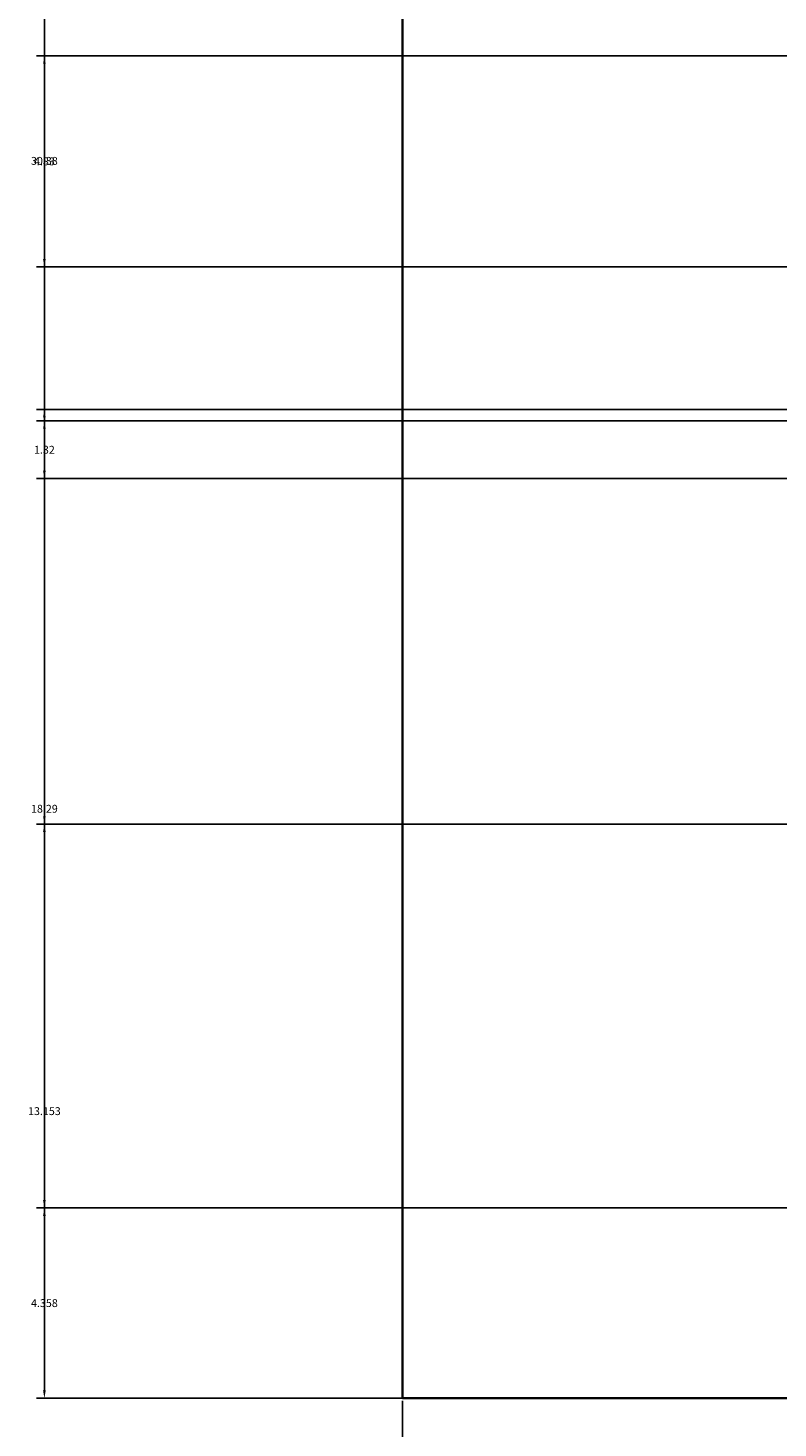
# Model space of a CAD drawing. Units: inches. Extents: x 27 to 200, y -50 to 102.
# Tile 2 of 26: x 27 to 44, y -17 to 15. Entities that reach past the tile are written whole.
import ezdxf

# ---------------------------------------------------------------- set-up
doc = ezdxf.new("R2010")
doc.units = ezdxf.units.IN
doc.header["$MEASUREMENT"] = 0
doc.layers.add('A-ANNO-DIMS', color=2, linetype='Continuous', lineweight=18)
doc.layers.add('A-ELEV', color=7, linetype='Continuous', lineweight=35)
doc.styles.get("Standard").update_dxf_attribs({"font": 'arial.ttf'})
doc.dimstyles.get("Standard").update_dxf_attribs({"dimtxt": 0.18, "dimasz": 0.18, "dimexe": 0.18, "dimexo": 0.0625, "dimgap": 0.09, "dimtad": 0, "dimtih": 1, "dimtoh": 1, "dimdec": 4, "dimzin": 0, "dimdsep": 46, "dimtxsty": 'Standard', "dimcen": 0.09, "dimadec": 0, "dimazin": 0, "dimtfac": 1, "dimtdec": 4, "dimtofl": 0, "dimtmove": 0, "dimatfit": 3, "dimfxl": 1, "dimtolj": 1, "dimtzin": 0, "dimarcsym": 0})

# ---------------------------------------------------------------- blocks, each defined once
blk = doc.blocks.new('*D23')
at = {"layer": 'A-ANNO-DIMS', "color": 0, "lineweight": -2, "transparency": 16777216}
for p, q in [((35.417, -16.832), (35.417, -25.149)), ((191.417, -16.832), (191.417, -25.149)), ((35.597, -24.969), (113.137, -24.969)), ((191.237, -24.969), (113.697, -24.969))]:
    blk.add_line(p, q, dxfattribs=at)
at = {"layer": 'A-ANNO-DIMS', "color": 0, "transparency": 16777216}
for points in [[(35.597, -24.939), (35.597, -24.999), (35.417, -24.969)], [(191.237, -24.939), (191.237, -24.999), (191.417, -24.969)]]:
    blk.add_solid(points, dxfattribs=at)
at = {"layer": 'Defpoints', "color": 0, "transparency": 16777216}
for p in [(35.417, -16.769), (191.417, -16.769), (191.417, -24.969)]:
    blk.add_point(p, dxfattribs=at)
at = {"layer": 'A-ANNO-DIMS', "color": 0, "transparency": 16777216, "insert": (113.417, -24.969), "char_height": 0.18, "attachment_point": 5}
blk.add_mtext('\\A1;156', dxfattribs=at)
blk = doc.blocks.new('*D24')
at = {"layer": 'A-ANNO-DIMS', "color": 0, "lineweight": -2, "transparency": 16777216}
for p, q in [((35.354, 93.926), (27.037, 93.926)), ((27.217, 93.746), (27.217, 38.76)), ((27.217, -16.589), (27.217, 38.397)), ((35.354, -16.769), (27.037, -16.769))]:
    blk.add_line(p, q, dxfattribs=at)
at = {"layer": 'A-ANNO-DIMS', "color": 0, "transparency": 16777216}
for points in [[(27.187, 93.746), (27.247, 93.746), (27.217, 93.926)], [(27.187, -16.589), (27.247, -16.589), (27.217, -16.769)]]:
    blk.add_solid(points, dxfattribs=at)
at = {"layer": 'Defpoints', "color": 0, "transparency": 16777216}
for p in [(27.217, 93.926), (35.417, 93.926), (35.417, -16.769)]:
    blk.add_point(p, dxfattribs=at)
at = {"layer": 'A-ANNO-DIMS', "color": 0, "transparency": 16777216, "insert": (27.217, 38.579), "char_height": 0.18, "attachment_point": 5}
blk.add_mtext('\\A1;110.7', dxfattribs=at)
blk = doc.blocks.new('*D44')
at = {"layer": 'A-ANNO-DIMS', "color": 0, "lineweight": -2, "transparency": 16777216}
for p, q in [((62.443, -3.617), (27.037, -3.617)), ((27.217, -3.797), (27.217, -10.011)), ((27.217, -16.589), (27.217, -10.375)), ((44.354, -16.769), (27.037, -16.769))]:
    blk.add_line(p, q, dxfattribs=at)
at = {"layer": 'A-ANNO-DIMS', "color": 0, "transparency": 16777216}
for points in [[(27.187, -3.797), (27.247, -3.797), (27.217, -3.617)], [(27.187, -16.589), (27.247, -16.589), (27.217, -16.769)]]:
    blk.add_solid(points, dxfattribs=at)
at = {"layer": 'Defpoints', "color": 0, "transparency": 16777216}
for p in [(27.217, -3.617), (62.505, -3.617), (44.417, -16.769)]:
    blk.add_point(p, dxfattribs=at)
at = {"layer": 'A-ANNO-DIMS', "color": 0, "transparency": 16777216, "insert": (27.217, -10.193), "char_height": 0.18, "attachment_point": 5}
blk.add_mtext('\\A1;13.153', dxfattribs=at)
blk = doc.blocks.new('*D45')
at = {"layer": 'A-ANNO-DIMS', "color": 0, "lineweight": -2, "transparency": 16777216}
for p, q in [((62.443, 26.764), (27.037, 26.764)), ((27.217, 26.584), (27.217, 11.755)), ((27.217, -3.437), (27.217, 11.392)), ((62.443, -3.617), (27.037, -3.617))]:
    blk.add_line(p, q, dxfattribs=at)
at = {"layer": 'A-ANNO-DIMS', "color": 0, "transparency": 16777216}
for points in [[(27.187, 26.584), (27.247, 26.584), (27.217, 26.764)], [(27.187, -3.437), (27.247, -3.437), (27.217, -3.617)]]:
    blk.add_solid(points, dxfattribs=at)
at = {"layer": 'Defpoints', "color": 0, "transparency": 16777216}
for p in [(27.217, 26.764), (62.505, 26.764), (62.505, -3.617)]:
    blk.add_point(p, dxfattribs=at)
at = {"layer": 'A-ANNO-DIMS', "color": 0, "transparency": 16777216, "insert": (27.217, 11.573), "char_height": 0.18, "attachment_point": 5}
blk.add_mtext('\\A1;30.38', dxfattribs=at)
blk = doc.blocks.new('*D54')
at = {"layer": 'A-ANNO-DIMS', "color": 0, "lineweight": -2, "transparency": 16777216}
for p, q in [((120.833, 13.977), (27.037, 13.977)), ((27.217, 13.797), (27.217, 11.743)), ((27.217, 9.324), (27.217, 11.379)), ((120.833, 9.144), (27.037, 9.144))]:
    blk.add_line(p, q, dxfattribs=at)
at = {"layer": 'A-ANNO-DIMS', "color": 0, "transparency": 16777216}
for points in [[(27.187, 13.797), (27.247, 13.797), (27.217, 13.977)], [(27.187, 9.324), (27.247, 9.324), (27.217, 9.144)]]:
    blk.add_solid(points, dxfattribs=at)
at = {"layer": 'Defpoints', "color": 0, "transparency": 16777216}
for p in [(27.217, 13.977), (120.895, 13.977), (120.895, 9.144)]:
    blk.add_point(p, dxfattribs=at)
at = {"layer": 'A-ANNO-DIMS', "color": 0, "transparency": 16777216, "insert": (27.217, 11.561), "char_height": 0.18, "attachment_point": 5}
blk.add_mtext('\\A1;4.83', dxfattribs=at)
blk = doc.blocks.new('*D56')
at = {"layer": 'A-ANNO-DIMS', "color": 0, "lineweight": -2, "transparency": 16777216}
for p, q in [((121.225, 5.878), (27.037, 5.878)), ((27.217, 5.698), (27.217, -3.085)), ((27.217, -12.231), (27.217, -3.448)), ((121.225, -12.411), (27.037, -12.411))]:
    blk.add_line(p, q, dxfattribs=at)
at = {"layer": 'A-ANNO-DIMS', "color": 0, "transparency": 16777216}
for points in [[(27.187, 5.698), (27.247, 5.698), (27.217, 5.878)], [(27.187, -12.231), (27.247, -12.231), (27.217, -12.411)]]:
    blk.add_solid(points, dxfattribs=at)
at = {"layer": 'Defpoints', "color": 0, "transparency": 16777216}
for p in [(27.217, 5.878), (121.288, 5.878), (121.288, -12.411)]:
    blk.add_point(p, dxfattribs=at)
at = {"layer": 'A-ANNO-DIMS', "color": 0, "transparency": 16777216, "insert": (27.217, -3.267), "char_height": 0.18, "attachment_point": 5}
blk.add_mtext('\\A1;18.29', dxfattribs=at)
blk = doc.blocks.new('*D68')
at = {"layer": 'A-ANNO-DIMS', "color": 0, "lineweight": -2, "transparency": 16777216}
for p, q in [((145.153, 5.617), (27.037, 5.617)), ((27.217, 5.437), (27.217, 5.138)), ((27.217, 4.476), (27.217, 4.774)), ((145.153, 4.296), (27.037, 4.296))]:
    blk.add_line(p, q, dxfattribs=at)
at = {"layer": 'A-ANNO-DIMS', "color": 0, "transparency": 16777216}
for points in [[(27.187, 5.437), (27.247, 5.437), (27.217, 5.617)], [(27.187, 4.476), (27.247, 4.476), (27.217, 4.296)]]:
    blk.add_solid(points, dxfattribs=at)
at = {"layer": 'Defpoints', "color": 0, "transparency": 16777216}
for p in [(27.217, 5.617), (145.216, 5.617), (145.216, 4.296)]:
    blk.add_point(p, dxfattribs=at)
at = {"layer": 'A-ANNO-DIMS', "color": 0, "transparency": 16777216, "insert": (27.217, 4.956), "char_height": 0.18, "attachment_point": 5}
blk.add_mtext('\\A1;1.32', dxfattribs=at)
blk = doc.blocks.new('*D69')
at = {"layer": 'A-ANNO-DIMS', "color": 0, "lineweight": -2, "transparency": 16777216}
for p, q in [((121.225, -12.411), (27.037, -12.411)), ((27.217, -12.591), (27.217, -14.408)), ((27.217, -16.589), (27.217, -14.772)), ((119.249, -16.769), (27.037, -16.769))]:
    blk.add_line(p, q, dxfattribs=at)
at = {"layer": 'A-ANNO-DIMS', "color": 0, "transparency": 16777216}
for points in [[(27.187, -12.591), (27.247, -12.591), (27.217, -12.411)], [(27.187, -16.589), (27.247, -16.589), (27.217, -16.769)]]:
    blk.add_solid(points, dxfattribs=at)
at = {"layer": 'Defpoints', "color": 0, "transparency": 16777216}
for p in [(27.217, -12.411), (121.288, -12.411), (119.312, -16.769)]:
    blk.add_point(p, dxfattribs=at)
at = {"layer": 'A-ANNO-DIMS', "color": 0, "transparency": 16777216, "insert": (27.217, -14.59), "char_height": 0.18, "attachment_point": 5}
blk.add_mtext('\\A1;4.358', dxfattribs=at)

msp = doc.modelspace()

# ---------------------------------------------------------------- linework, layer by layer
at = {"layer": 'A-ELEV'}
for p, q in [((35.4169, 93.9264), (35.4169, -16.7693)), ((35.4169, -16.7693), (191.4169, -16.7693))]:
    msp.add_line(p, q, dxfattribs=at)

# ---------------------------------------------------------------- dimensions: what is measured, and where the dimension line sits
at = {"layer": 'A-ANNO-DIMS'}
for base, p1, p2, override, picture, middle in [((27.2169, 93.9264), (35.4169, -16.7693), (35.4169, 93.9264), {"dimdec": 1, "dimlfac": 1, "dimrnd": 0, "dimzin": 0, "dimdsep": 46, "dimlunit": 2}, '*D24', (27.2169, 38.5786)), ((27.2169, 26.7638), (62.5054, -3.6168), (62.5054, 26.7638), {"dimdec": 2, "dimlfac": 1, "dimrnd": 0, "dimzin": 0, "dimdsep": 46, "dimlunit": 2}, '*D45', (27.2169, 11.5735)), ((27.2169, 13.9773), (120.8954, 9.1438), (120.8954, 13.9773), {"dimdec": 2, "dimlfac": 1, "dimrnd": 0, "dimzin": 0, "dimdsep": 46, "dimlunit": 2}, '*D54', (27.2169, 11.5606)), ((27.2169, 5.8779), (121.2876, -12.411), (121.2876, 5.8779), {"dimdec": 2, "dimlfac": 1, "dimrnd": 0, "dimzin": 0, "dimdsep": 46, "dimlunit": 2}, '*D56', (27.2169, -3.2665)), ((27.2169, 5.6167), (145.216, 4.2959), (145.216, 5.6167), {"dimdec": 2, "dimlfac": 1, "dimrnd": 0, "dimzin": 0, "dimdsep": 46, "dimlunit": 2}, '*D68', (27.2169, 4.9563)), ((27.216902, -3.61681), (44.416902, -16.76931), (62.505395, -3.61681), {"dimdec": 3, "dimlfac": 1, "dimrnd": 0, "dimzin": 0, "dimdsep": 46, "dimlunit": 2}, '*D44', (27.216902, -10.19306)), ((27.2169, -12.411), (119.3118, -16.7693), (121.2876, -12.411), {"dimdec": 3, "dimlfac": 1, "dimrnd": 0, "dimzin": 0, "dimdsep": 46, "dimlunit": 2}, '*D69', (27.2169, -14.5901))]:
    dim = msp.add_linear_dim(base=base, p1=p1, p2=p2, angle=90, dimstyle='Standard', override=override, dxfattribs=at)
    dim.commit()
    dim.dimension.update_dxf_attribs({"geometry": picture, "text_midpoint": middle})
dim = msp.add_linear_dim(base=(191.4169, -24.9693), p1=(35.4169, -16.7693), p2=(191.4169, -16.7693), dimstyle='Standard', override={"dimdec": 0, "dimlfac": 1, "dimrnd": 0, "dimzin": 0, "dimdsep": 46, "dimlunit": 2}, dxfattribs=at)
dim.commit()
dim.dimension.update_dxf_attribs({"geometry": '*D23', "text_midpoint": (113.4169, -24.9693)})

doc.saveas('drawing.dxf')
